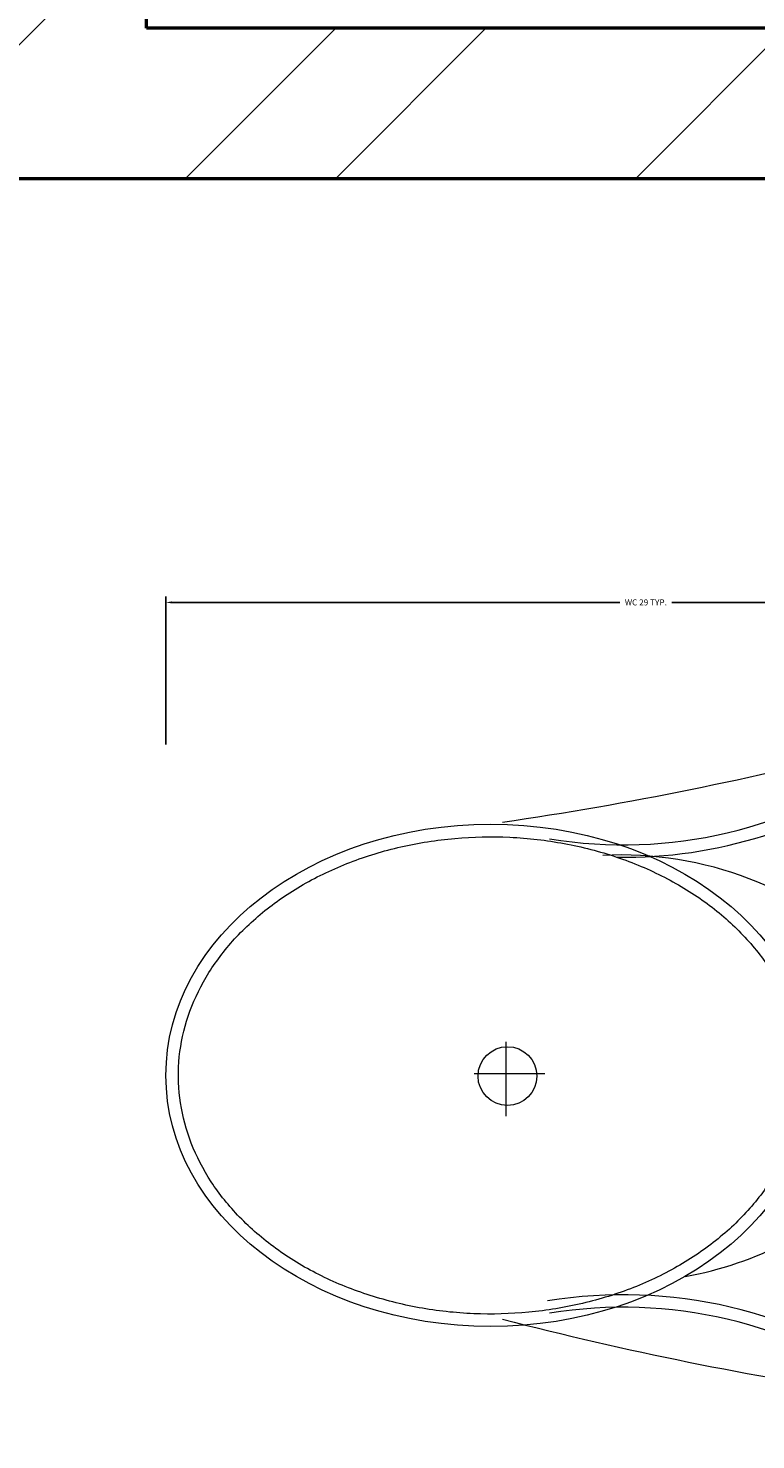
# Model space of a CAD drawing. Units: inches. Extents: x 963 to 2075, y 289 to 2657.
# Tile 34 of 98: x 1646 to 1668, y 1505 to 1547. Entities that reach past the tile are written whole.
import ezdxf

# ---------------------------------------------------------------- set-up
doc = ezdxf.new("R2010")
doc.units = ezdxf.units.IN
for name, color, linetype, lineweight in [('A-ANNO-DIMS', 2, 'Continuous', 18), ('A-FLOR-FIXT', 9, 'Continuous', 18), ('A-WALL', 7, 'Continuous', 50), ('A-WALL-PATT', 8, 'Continuous', 13)]:
    doc.layers.add(name, color=color, linetype=linetype, lineweight=lineweight)
doc.styles.get("Standard").update_dxf_attribs({"font": 'arial.ttf'})
doc.dimstyles.get("Standard").update_dxf_attribs({"dimtxt": 0.18, "dimasz": 0.18, "dimexe": 0.18, "dimexo": 0.0625, "dimgap": 0.09, "dimtad": 0, "dimtih": 1, "dimtoh": 1, "dimdec": 4, "dimzin": 0, "dimdsep": 46, "dimtxsty": 'Standard', "dimcen": 0.09, "dimadec": 0, "dimazin": 0, "dimtfac": 1, "dimtdec": 4, "dimtofl": 0, "dimtmove": 0, "dimatfit": 3, "dimfxl": 1, "dimtolj": 1, "dimtzin": 0, "dimarcsym": 0})

# ---------------------------------------------------------------- blocks, each defined once
blk = doc.blocks.new('A$C31115884')
for p, q in [((257.5, 466.4), (257.5, 523.2)), ((283.1, 497.7), (223.4, 497.7)), ((0, 200), (0, 0)), ((520, 200), (0, 200)), ((520, 0), (520, 200)), ((10, 190), (10, 10)), ((510, 190), (10, 190)), ((510, 10), (510, 190)), ((510, 54.5), (0, 54.5)), ((10, 10), (510, 10)), ((0, 0), (520, 0))]:
    blk.add_line(p, q)
blk.add_circle((255.6, 496.4), 23.6)
for centre, radius, start, end in [((2777.7, -204.6), 2807, 165.4549, 171.7133), ((3237, 905), 2807, 188.2867, 194.5451), ((-294.5, 403.3), 364.7, 324.2091, 9.3499), ((-294.5, 403.3), 374.7, 324.2091, 9.3499), ((805.8, 403.3), 364.7, 170.6501, 215.7909), ((139.5, 406.2), 293.5, 315.8436, 2.6563), ((805.8, 403.3), 374.7, 179.2036, 215.7909), ((383.6, 406.2), 293.5, 190.2774, 224.1564)]:
    blk.add_arc(centre, radius, start, end)
blk.add_ellipse((256.2, 509.9), major_axis=(0, -260.7), ratio=0.772727)
blk.add_open_spline([(256.2, 259.2), (263.1, 259.2), (270, 259.7), (287.8, 262.3), (298.7, 265.1), (319.9, 273.1), (330.2, 278.4), (350.1, 291.1), (359.7, 298.7), (377.7, 315.9), (386.2, 325.5), (401.7, 346.6), (408.8, 358.1), (421.3, 382.5), (426.8, 395.5), (435.9, 422.4), (439.5, 436.4), (444.8, 465.1), (446.5, 479.7), (447.9, 509.2), (447.6, 524), (445, 553.3), (442.7, 567.8), (436.3, 596), (432.1, 609.7), (421.9, 636), (416, 648.6), (402.5, 672.1), (395, 683), (378.6, 703), (369.8, 712.1), (351.1, 728), (341.3, 734.8), (320.9, 746.2), (310.4, 750.7), (288.9, 757.3), (278, 759.4), (256, 761), (245, 760.6), (223.1, 757.2), (212.3, 754.3), (191.1, 746.1), (180.8, 740.7), (160.9, 727.8), (151.4, 720.1), (133.5, 702.7), (125.1, 693), (109.6, 671.7), (102.6, 660.2), (90.2, 635.7), (84.9, 622.7), (76, 595.6), (72.4, 581.6), (67.2, 552.9), (65.6, 538.2), (64.4, 508.8), (64.8, 494), (67.5, 464.7), (69.9, 450.2), (76.6, 422), (80.8, 408.3), (91.1, 382.2), (97.2, 369.7), (110.8, 346.3), (118.4, 335.4), (134.8, 315.6), (143.7, 306.7), (162.4, 290.9), (172.3, 284.2), (192.8, 273), (203.3, 268.6), (224.8, 262.2), (235.8, 260.2), (249.9, 259.3), (253, 259.2), (256.2, 259.2)], degree=3, knots=[0, 0, 0, 0, 0.110105, 0.110105, 0.285049, 0.285049, 0.459994, 0.459994, 0.634938, 0.634938, 0.809882, 0.809882, 0.984827, 0.984827, 1.159771, 1.159771, 1.334715, 1.334715, 1.50966, 1.50966, 1.684604, 1.684604, 1.859549, 1.859549, 2.034493, 2.034493, 2.209437, 2.209437, 2.384382, 2.384382, 2.559326, 2.559326, 2.73427, 2.73427, 2.909215, 2.909215, 3.084159, 3.084159, 3.259103, 3.259103, 3.434048, 3.434048, 3.608992, 3.608992, 3.783936, 3.783936, 3.958881, 3.958881, 4.133825, 4.133825, 4.30877, 4.30877, 4.483714, 4.483714, 4.658658, 4.658658, 4.833603, 4.833603, 5.008547, 5.008547, 5.183491, 5.183491, 5.358436, 5.358436, 5.53338, 5.53338, 5.708324, 5.708324, 5.883269, 5.883269, 6.058213, 6.058213, 6.233158, 6.233158, 6.283185, 6.283185, 6.283185, 6.283185])
blk = doc.blocks.new('*D16')
at = {"layer": 'A-ANNO-DIMS', "color": 0, "lineweight": -2, "transparency": 16777216}
for p, q in [((1650.002, 1525.905), (1650.002, 1530.33)), ((1678.722, 1525.905), (1678.722, 1530.33)), ((1650.182, 1530.15), (1663.586, 1530.15)), ((1678.542, 1530.15), (1665.138, 1530.15))]:
    blk.add_line(p, q, dxfattribs=at)
at = {"layer": 'A-ANNO-DIMS', "color": 0, "transparency": 16777216}
for points in [[(1650.182, 1530.18), (1650.182, 1530.12), (1650.002, 1530.15)], [(1678.542, 1530.18), (1678.542, 1530.12), (1678.722, 1530.15)]]:
    blk.add_solid(points, dxfattribs=at)
at = {"layer": 'Defpoints', "color": 0, "transparency": 16777216}
for p in [(1650.002, 1530.15), (1650.002, 1525.842), (1678.722, 1525.842)]:
    blk.add_point(p, dxfattribs=at)
at = {"layer": 'A-ANNO-DIMS', "color": 0, "transparency": 16777216, "insert": (1664.362, 1530.15), "char_height": 0.18, "attachment_point": 5}
blk.add_mtext('\\A1;WC 29 TYP.', dxfattribs=at)

msp = doc.modelspace()

# ---------------------------------------------------------------- hatches: boundary and pattern name
at = {"layer": 'A-WALL-PATT'}
h = msp.add_hatch(dxfattribs=at)
h.set_pattern_fill('ANSI32', color=256)
h.paths.add_polyline_path([(1910.422, 1929.422), (1910.422, 1963.511), (1905.922, 1963.511), (1905.922, 1929.422), (1845.922, 1929.422), (1845.922, 1993.365), (1843.672, 1993.365), (1841.422, 1993.365), (1841.422, 1951.163), (1841.422, 1924.922), (1853.422, 1924.922), (1853.422, 1913.074), (1857.922, 1913.074), (1857.922, 1924.922), (1910.422, 1924.922)])
h.paths.add_polyline_path([(1857.922, 1853.074), (1853.422, 1853.074), (1853.422, 1826.318), (1841.422, 1826.318), (1674.482, 1826.318), (1674.482, 1821.818), (1853.422, 1821.818), (1857.922, 1821.818)])
h.paths.add_polyline_path([(1857.922, 1821.818), (1853.422, 1821.818), (1853.422, 1807.793), (1857.922, 1807.793)])
h.paths.add_polyline_path([(1857.922, 1747.793), (1853.422, 1747.793), (1853.422, 1713.818), (1809.343, 1713.818), (1809.343, 1709.318), (1905.922, 1709.318), (1905.922, 1688.318), (1910.422, 1688.318), (1910.422, 1713.818), (1857.922, 1713.818)])
h.paths.add_polyline_path([(1830.922, 1542.818), (1837.429, 1542.818), (1837.429, 1545.068), (1837.429, 1547.318), (1823.419, 1547.318), (1823.419, 1545.068), (1823.419, 1542.818), (1826.422, 1542.818), (1826.422, 1482.818), (1742.422, 1482.818), (1742.422, 1505.389), (1737.922, 1505.389), (1737.922, 1478.318), (1830.922, 1478.318)])
h.paths.add_polyline_path([(1938.922, 1619.318), (1934.422, 1619.318), (1910.422, 1619.318), (1910.422, 1628.318), (1908.172, 1628.318), (1905.922, 1628.318), (1905.922, 1614.818), (1934.422, 1614.818), (1934.422, 1547.318), (1905.922, 1547.318), (1899.589, 1547.318), (1899.589, 1542.818), (1910.422, 1542.818), (1938.922, 1542.818)])
h.paths.add_polyline_path([(1803.676, 1547.318), (1773.922, 1547.318), (1773.922, 1709.318), (1777.757, 1709.318), (1777.757, 1713.818), (1701.922, 1713.818), (1701.922, 1697.802), (1706.422, 1697.802), (1706.422, 1709.318), (1769.422, 1709.318), (1769.422, 1662.818), (1706.422, 1662.818), (1706.422, 1674.385), (1701.922, 1674.385), (1701.922, 1662.818), (1675.672, 1662.818), (1675.672, 1658.318), (1769.422, 1658.318), (1769.422, 1547.318), (1729.17, 1547.318), (1729.17, 1542.818), (1737.922, 1542.818), (1737.922, 1529.389), (1742.422, 1529.389), (1742.422, 1542.818), (1803.676, 1542.818)])
h.paths.add_polyline_path([(1595.422, 1542.818), (1599.245, 1542.818), (1599.245, 1547.318), (1584.36, 1547.318), (1584.36, 1542.818), (1590.922, 1542.818), (1590.922, 1436.318), (1595.422, 1436.318), (1595.422, 1440.818)])
h.paths.add_polyline_path([(1693.17, 1547.318), (1649.422, 1547.318), (1649.422, 1658.318), (1652.098, 1658.318), (1652.098, 1660.568), (1652.098, 1662.818), (1649.422, 1662.818), (1649.422, 1680.937), (1647.172, 1680.937), (1644.922, 1680.937), (1644.922, 1547.318), (1622.422, 1547.318), (1622.422, 1545.068), (1622.422, 1542.818), (1649.422, 1542.818), (1679.422, 1542.818), (1679.422, 1529.845), (1681.672, 1529.845), (1683.922, 1529.845), (1683.922, 1542.818), (1693.17, 1542.818), (1693.17, 1545.068)])
h.paths.add_polyline_path([(1683.922, 1505.845), (1679.422, 1505.845), (1679.422, 1483.805), (1595.422, 1483.805), (1595.422, 1479.305), (1683.922, 1479.305)])
h.paths.add_polyline_path([(1402.993, 1547.318), (1376.422, 1547.318), (1376.422, 1675.888), (1374.172, 1675.888), (1371.922, 1675.888), (1371.922, 1662.818), (1368.876, 1662.818), (1368.876, 1658.318), (1371.922, 1658.318), (1371.922, 1547.318), (1335.464, 1547.318), (1335.464, 1542.818), (1337.422, 1542.818), (1337.422, 1526.732), (1341.922, 1526.732), (1341.922, 1542.818), (1371.922, 1542.818), (1402.993, 1542.818)])

# ---------------------------------------------------------------- linework, layer by layer
at = {"layer": 'A-WALL'}
for p, q in [((1649.422, 1547.318), (1649.422, 1658.318)), ((1693.17, 1547.318), (1649.422, 1547.318)), ((1649.422, 1542.818), (1620.795, 1542.818)), ((1679.422, 1542.818), (1649.422, 1542.818))]:
    msp.add_line(p, q, dxfattribs=at)

# ---------------------------------------------------------------- block references
at = {"layer": 'A-FLOR-FIXT', "xscale": 0.0372717239612423, "yscale": 0.0372717239612423, "zscale": 0.0372717239612423, "rotation": 89.99999999999999}
msp.add_blockref('A$C31115884', (1678.722, 1506.461), dxfattribs=at)

# ---------------------------------------------------------------- dimensions: what is measured, and where the dimension line sits
at = {"layer": 'A-ANNO-DIMS'}
dim = msp.add_linear_dim(base=(1650.002, 1530.15), p1=(1678.722, 1525.842), p2=(1650.002, 1525.842), angle=180, text='WC <> TYP.', dimstyle='Standard', override={"dimdec": 0, "dimlfac": 1, "dimrnd": 0, "dimzin": 0, "dimdsep": 46, "dimlunit": 2}, dxfattribs=at)
dim.commit()
dim.dimension.update_dxf_attribs({"geometry": '*D16', "text_midpoint": (1664.362, 1530.15)})

doc.saveas('drawing.dxf')
